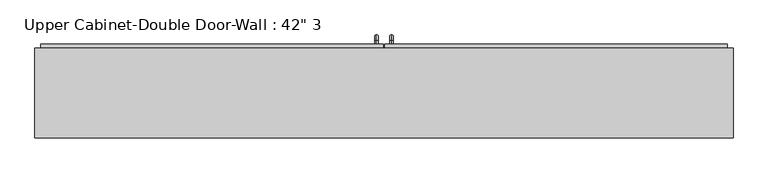
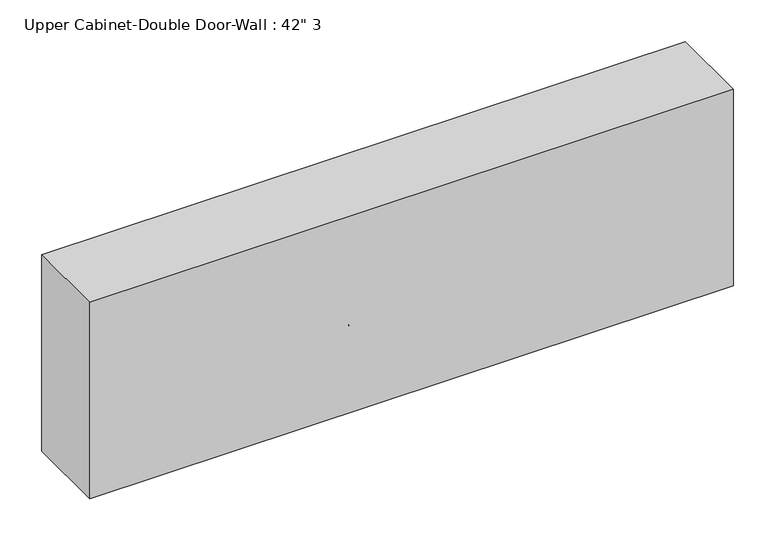
"""IFC4 building model written with IfcOpenShell, lengths in millimetres: furniture geometry."""

from ifc_helpers import new_model, si_unit, point, frame, origin, place, context, project, spatial, polyline, circle_curve, ellipse_curve, trimmed, outline, extrude, faceted_brep, source, transform, mapped, element, save
from ifc_brep_helpers import plane_surface, cylinder_surface, revolved_surface, advanced_brep


def furniture_3df5d44a(model_context):
    return source(origin(), model_context, "Body", "SolidModel", [
        extrude(outline(polyline([(32.9461628, 431.8), (1191.8211628, 431.8), (1191.8211628, 400.05), (32.9461628, 400.05), (32.9461628, 431.8)])), frame((0.0, 0.0, 1390.65), z_axis=(0.0, 0.0, 1.0), x_axis=(1.0, 0.0, 0.0)), (0.0, 0.0, 1.0), 723.9),
        extrude(outline(polyline([(-1132.2788372, 431.8), (26.5961628, 431.8), (26.5961628, 400.05), (-1132.2788372, 400.05), (-1132.2788372, 431.8)])), frame((0.0, 0.0, 1390.65), z_axis=(0.0, 0.0, 1.0), x_axis=(1.0, 0.0, 0.0)), (0.0, 0.0, 1.0), 723.9),
        advanced_brep(
        [(4.3711628, 431.8, 1517.65), (4.3711628, 431.8, 1530.35), (4.3711628, 444.5, 1517.65), (4.3711628, 444.5, 1530.35), (4.3711628, 463.55, 1511.3), (4.3711628, 450.85, 1511.3), (4.3711628, 450.85, 1435.1), (4.3711628, 463.55, 1435.1), (4.3711628, 444.5, 1416.05), (4.3711628, 444.5, 1428.75), (4.3711628, 431.8, 1428.75), (4.3711628, 431.8, 1416.05)],
        [
            (0, 1, circle_curve(frame((4.3711628, 431.8, 1524.0), z_axis=(0.0, -1.0, 0.0), x_axis=(0.0, 0.0, 1.0)), 6.35)),
            (1, 0, circle_curve(frame((4.3711628, 431.8, 1524.0), z_axis=(0.0, -1.0, 0.0), x_axis=(0.0, 0.0, 1.0)), 6.35)),
            (0, 2),
            (2, 3, circle_curve(frame((4.3711628, 444.5, 1524.0), z_axis=(0.0, -1.0, 0.0), x_axis=(0.0, 0.0, 1.0)), 6.35)),
            (3, 1),
            (3, 2, circle_curve(frame((4.3711628, 444.5, 1524.0), z_axis=(0.0, -1.0, 0.0), x_axis=(0.0, 0.0, 1.0)), 6.35)),
            (4, 3, circle_curve(frame((4.3711628, 444.5, 1511.3), z_axis=(1.0, 0.0, 0.0), x_axis=(0.0, 0.0, 1.0)), 19.05)),
            (2, 5, circle_curve(frame((4.3711628, 444.5, 1511.3), z_axis=(-1.0, 0.0, 0.0), x_axis=(0.0, 0.0, 1.0)), 6.35)),
            (5, 4, circle_curve(frame((4.3711628, 457.2, 1511.3), z_axis=(0.0, 0.0, 1.0), x_axis=(0.0, 1.0, 0.0)), 6.35)),
            (4, 5, circle_curve(frame((4.3711628, 457.2, 1511.3), z_axis=(0.0, 0.0, 1.0), x_axis=(0.0, 1.0, 0.0)), 6.35)),
            (5, 6),
            (6, 7, circle_curve(frame((4.3711628, 457.2, 1435.1), z_axis=(0.0, 0.0, 1.0), x_axis=(0.0, 1.0, 0.0)), 6.35)),
            (7, 4),
            (7, 6, circle_curve(frame((4.3711628, 457.2, 1435.1), z_axis=(0.0, 0.0, 1.0), x_axis=(0.0, 1.0, 0.0)), 6.35)),
            (8, 7, circle_curve(frame((4.3711628, 444.5, 1435.1), z_axis=(1.0, 0.0, 0.0), x_axis=(0.0, 1.0, 0.0)), 19.05)),
            (6, 9, circle_curve(frame((4.3711628, 444.5, 1435.1), z_axis=(-1.0, 0.0, 0.0), x_axis=(0.0, 1.0, 0.0)), 6.35)),
            (9, 8, circle_curve(frame((4.3711628, 444.5, 1422.4), z_axis=(0.0, 1.0, 0.0), x_axis=(0.0, 0.0, -1.0)), 6.35)),
            (8, 9, circle_curve(frame((4.3711628, 444.5, 1422.4), z_axis=(0.0, 1.0, 0.0), x_axis=(0.0, 0.0, -1.0)), 6.35)),
            (10, 11, circle_curve(frame((4.3711628, 431.8, 1422.4), z_axis=(0.0, -1.0, 0.0), x_axis=(0.0, 0.0, -1.0)), 6.35)),
            (11, 10, circle_curve(frame((4.3711628, 431.8, 1422.4), z_axis=(0.0, -1.0, 0.0), x_axis=(0.0, 0.0, -1.0)), 6.35)),
            (9, 10),
            (11, 8),
        ],
        [
            plane_surface(frame((-1.9788372, 431.8, 1524.0), z_axis=(0.0, -1.0, 0.0), x_axis=(0.0, 0.0, 1.0))),
            cylinder_surface(frame((4.3711628, 431.8, 1524.0), z_axis=(0.0, -1.0, 0.0), x_axis=(0.0, 0.0, 1.0)), 6.35),
            revolved_surface(trimmed(ellipse_curve(frame((4.3711628, 444.5, 1524.0), z_axis=(0.0, -1.0, 0.0), x_axis=(0.0, 0.0, 1.0)), 6.35, 6.35), [point((4.3711628, 444.5, 1517.65))], [point((4.3711628, 444.5, 1530.35))], True, "CARTESIAN"), (4.3711628, 444.5, 1511.3), (-1.0, 0.0, 0.0)),
            revolved_surface(trimmed(ellipse_curve(frame((4.3711628, 444.5, 1524.0), z_axis=(0.0, -1.0, 0.0), x_axis=(0.0, 0.0, 1.0)), 6.35, 6.35), [point((4.3711628, 444.5, 1530.35))], [point((4.3711628, 444.5, 1517.65))], True, "CARTESIAN"), (4.3711628, 444.5, 1511.3), (-1.0, 0.0, 0.0)),
            cylinder_surface(frame((4.3711628, 457.2, 1511.3), z_axis=(0.0, 0.0, 1.0), x_axis=(0.0, 1.0, 0.0)), 6.35),
            revolved_surface(trimmed(ellipse_curve(frame((4.3711628, 457.2, 1435.1), z_axis=(0.0, 0.0, 1.0), x_axis=(0.0, 1.0, 0.0)), 6.35, 6.35), [point((4.3711628, 450.85, 1435.1))], [point((4.3711628, 463.55, 1435.1))], True, "CARTESIAN"), (4.3711628, 444.5, 1435.1), (-1.0, 0.0, 0.0)),
            revolved_surface(trimmed(ellipse_curve(frame((4.3711628, 457.2, 1435.1), z_axis=(0.0, 0.0, 1.0), x_axis=(0.0, 1.0, 0.0)), 6.35, 6.35), [point((4.3711628, 463.55, 1435.1))], [point((4.3711628, 450.85, 1435.1))], True, "CARTESIAN"), (4.3711628, 444.5, 1435.1), (-1.0, 0.0, 0.0)),
            plane_surface(frame((-1.9788372, 431.8, 1422.4), z_axis=(0.0, -1.0, 0.0), x_axis=(0.0, 0.0, -1.0))),
            cylinder_surface(frame((4.3711628, 444.5, 1422.4), z_axis=(0.0, 1.0, 0.0), x_axis=(0.0, 0.0, -1.0)), 6.35),
        ],
        [
            (0, [[1, 2]]),
            (1, [[-1, 3, 4, 5]]),
            (1, [[-2, -5, 6, -3]]),
            (2, [[7, -4, 8, 9]]),
            (3, [[-8, -6, -7, 10]]),
            (4, [[-9, 11, 12, 13]]),
            (4, [[-10, -13, 14, -11]]),
            (5, [[15, -12, 16, 17]]),
            (6, [[-16, -14, -15, 18]]),
            (7, [[19, 20]]),
            (8, [[-17, 21, -20, 22]]),
            (8, [[-18, -22, -19, -21]]),
        ],
    ),
        advanced_brep(
        [(55.1711628, 431.8, 1517.65), (55.1711628, 431.8, 1530.35), (55.1711628, 444.5, 1517.65), (55.1711628, 444.5, 1530.35), (55.1711628, 463.55, 1511.3), (55.1711628, 450.85, 1511.3), (55.1711628, 450.85, 1435.1), (55.1711628, 463.55, 1435.1), (55.1711628, 444.5, 1416.05), (55.1711628, 444.5, 1428.75), (55.1711628, 431.8, 1428.75), (55.1711628, 431.8, 1416.05)],
        [
            (0, 1, circle_curve(frame((55.1711628, 431.8, 1524.0), z_axis=(0.0, -1.0, 0.0), x_axis=(0.0, 0.0, -1.0)), 6.35)),
            (1, 0, circle_curve(frame((55.1711628, 431.8, 1524.0), z_axis=(0.0, -1.0, 0.0), x_axis=(0.0, 0.0, -1.0)), 6.35)),
            (0, 2),
            (2, 3, circle_curve(frame((55.1711628, 444.5, 1524.0), z_axis=(0.0, -1.0, 0.0), x_axis=(0.0, 0.0, -1.0)), 6.35)),
            (3, 1),
            (3, 2, circle_curve(frame((55.1711628, 444.5, 1524.0), z_axis=(0.0, -1.0, 0.0), x_axis=(0.0, 0.0, -1.0)), 6.35)),
            (4, 3, circle_curve(frame((55.1711628, 444.5, 1511.3), z_axis=(1.0, 0.0, 0.0), x_axis=(0.0, 0.0, 1.0)), 19.05)),
            (2, 5, circle_curve(frame((55.1711628, 444.5, 1511.3), z_axis=(-1.0, 0.0, 0.0), x_axis=(0.0, 0.0, 1.0)), 6.35)),
            (5, 4, circle_curve(frame((55.1711628, 457.2, 1511.3), z_axis=(0.0, 0.0, 1.0), x_axis=(0.0, -1.0, 0.0)), 6.35)),
            (4, 5, circle_curve(frame((55.1711628, 457.2, 1511.3), z_axis=(0.0, 0.0, 1.0), x_axis=(0.0, -1.0, 0.0)), 6.35)),
            (5, 6),
            (6, 7, circle_curve(frame((55.1711628, 457.2, 1435.1), z_axis=(0.0, 0.0, 1.0), x_axis=(0.0, -1.0, 0.0)), 6.35)),
            (7, 4),
            (7, 6, circle_curve(frame((55.1711628, 457.2, 1435.1), z_axis=(0.0, 0.0, 1.0), x_axis=(0.0, -1.0, 0.0)), 6.35)),
            (8, 7, circle_curve(frame((55.1711628, 444.5, 1435.1), z_axis=(1.0, 0.0, 0.0), x_axis=(0.0, 1.0, 0.0)), 19.05)),
            (6, 9, circle_curve(frame((55.1711628, 444.5, 1435.1), z_axis=(-1.0, 0.0, 0.0), x_axis=(0.0, 1.0, 0.0)), 6.35)),
            (9, 8, circle_curve(frame((55.1711628, 444.5, 1422.4), z_axis=(0.0, 1.0, 0.0), x_axis=(0.0, 0.0, 1.0)), 6.35)),
            (8, 9, circle_curve(frame((55.1711628, 444.5, 1422.4), z_axis=(0.0, 1.0, 0.0), x_axis=(0.0, 0.0, 1.0)), 6.35)),
            (10, 11, circle_curve(frame((55.1711628, 431.8, 1422.4), z_axis=(0.0, -1.0, 0.0), x_axis=(0.0, 0.0, 1.0)), 6.35)),
            (11, 10, circle_curve(frame((55.1711628, 431.8, 1422.4), z_axis=(0.0, -1.0, 0.0), x_axis=(0.0, 0.0, 1.0)), 6.35)),
            (9, 10),
            (11, 8),
        ],
        [
            plane_surface(frame((48.8211628, 431.8, 1524.0), z_axis=(0.0, -1.0, 0.0), x_axis=(0.0, 0.0, 1.0))),
            cylinder_surface(frame((55.1711628, 431.8, 1524.0), z_axis=(0.0, -1.0, 0.0), x_axis=(0.0, 0.0, -1.0)), 6.35),
            revolved_surface(trimmed(ellipse_curve(frame((55.1711628, 444.5, 1524.0), z_axis=(0.0, -1.0, 0.0), x_axis=(0.0, 0.0, -1.0)), 6.35, 6.35), [point((55.1711628, 444.5, 1517.65))], [point((55.1711628, 444.5, 1530.35))], True, "CARTESIAN"), (55.1711628, 444.5, 1511.3), (-1.0, 0.0, 0.0)),
            revolved_surface(trimmed(ellipse_curve(frame((55.1711628, 444.5, 1524.0), z_axis=(0.0, -1.0, 0.0), x_axis=(0.0, 0.0, -1.0)), 6.35, 6.35), [point((55.1711628, 444.5, 1530.35))], [point((55.1711628, 444.5, 1517.65))], True, "CARTESIAN"), (55.1711628, 444.5, 1511.3), (-1.0, 0.0, 0.0)),
            cylinder_surface(frame((55.1711628, 457.2, 1511.3), z_axis=(0.0, 0.0, 1.0), x_axis=(0.0, -1.0, 0.0)), 6.35),
            revolved_surface(trimmed(ellipse_curve(frame((55.1711628, 457.2, 1435.1), z_axis=(0.0, 0.0, 1.0), x_axis=(0.0, -1.0, 0.0)), 6.35, 6.35), [point((55.1711628, 450.85, 1435.1))], [point((55.1711628, 463.55, 1435.1))], True, "CARTESIAN"), (55.1711628, 444.5, 1435.1), (-1.0, 0.0, 0.0)),
            revolved_surface(trimmed(ellipse_curve(frame((55.1711628, 457.2, 1435.1), z_axis=(0.0, 0.0, 1.0), x_axis=(0.0, -1.0, 0.0)), 6.35, 6.35), [point((55.1711628, 463.55, 1435.1))], [point((55.1711628, 450.85, 1435.1))], True, "CARTESIAN"), (55.1711628, 444.5, 1435.1), (-1.0, 0.0, 0.0)),
            plane_surface(frame((48.8211628, 431.8, 1422.4), z_axis=(0.0, -1.0, 0.0), x_axis=(0.0, 0.0, -1.0))),
            cylinder_surface(frame((55.1711628, 444.5, 1422.4), z_axis=(0.0, 1.0, 0.0), x_axis=(0.0, 0.0, 1.0)), 6.35),
        ],
        [
            (0, [[1, 2]]),
            (1, [[-1, 3, 4, 5]]),
            (1, [[-2, -5, 6, -3]]),
            (2, [[7, -4, 8, 9]]),
            (3, [[-8, -6, -7, 10]]),
            (4, [[-9, 11, 12, 13]]),
            (4, [[-10, -13, 14, -11]]),
            (5, [[15, -12, 16, 17]]),
            (6, [[-16, -14, -15, 18]]),
            (7, [[19, 20]]),
            (8, [[-17, 21, -20, 22]]),
            (8, [[-18, -22, -19, -21]]),
        ],
    ),
        faceted_brep([(-1151.3288372, 114.3, 2133.6), (-1151.3288372, 114.3, 1371.6), (1210.8711628, 114.3, 1371.6), (1210.8711628, 114.3, 2133.6), (-1151.3288372, 419.1, 2133.6), (1210.8711628, 419.1, 2133.6), (1210.8711628, 419.1, 1371.6), (-1151.3288372, 419.1, 1371.6), (-1132.2788372, 419.1, 2114.55), (-1132.2788372, 419.1, 1390.65), (1191.8211628, 419.1, 1390.65), (1191.8211628, 419.1, 2114.55), (1191.8211628, 133.35, 2114.55), (-1132.2788372, 133.35, 2114.55), (1191.8211628, 133.35, 1390.65), (-1132.2788372, 133.35, 1390.65)], [[[0, 1, 2, 3]], [[4, 5, 6, 7], [8, 9, 10, 11]], [[1, 0, 4, 7]], [[2, 1, 7, 6]], [[3, 2, 6, 5]], [[0, 3, 5, 4]], [[8, 11, 12, 13]], [[11, 10, 14, 12]], [[10, 9, 15, 14]], [[9, 8, 13, 15]], [[13, 12, 14, 15]]]),
    ])


if __name__ == "__main__":
    model = new_model("IFC4")
    model_context = context("Model", 3, world=origin())
    ifc_project = project(units=[si_unit("LENGTHUNIT", "METRE", prefix="MILLI")], contexts=[model_context])
    site = spatial("IfcSite", under=ifc_project)
    building = spatial("IfcBuilding", under=site)
    placement = place(None, origin())
    furniture_shape = furniture_3df5d44a(model_context)
    element("IfcFurniture", 1, ObjectType="Upper Cabinet-Double Door-Wall : 42\" 3", at=placement, inside=building, context=model_context, shape_type="MappedRepresentation", body=[
        mapped(furniture_shape, transform((0.0, 0.0, 0.0), x_axis=(1.0, 0.0, 0.0), y_axis=(0.0, 1.0, 0.0), z_axis=(0.0, 0.0, 1.0))),
    ])
    save(model, "model.ifc")

# Revit data of these elements
# Type "Upper Cabinet-Double Door-Wall : 42\" 3"
#   Assembly Code = "C1030410"
#   Depth = 1' - 0"
#   Height = 2' - 6"
#   Top Of Cabinet = 7' - 0"
#   Width = 7' - 9"
#   Cabinet Material = none
#   Door/Drawer Material = none
#   Handle Material = Cabinets - Handles
#   Default Elevation = 0
# Element 1 (IfcFurniture, "Upper Cabinet-Double Door-Wall : 42\" 3")
#   Materials on its faces: "Cabinets - Handles", "Cabinet"
# Materials
#   "Cabinets - Handles": colour RGB 57 57 57, transparency 0
#   "Cabinet": colour RGB 204 122 2, transparency 0
